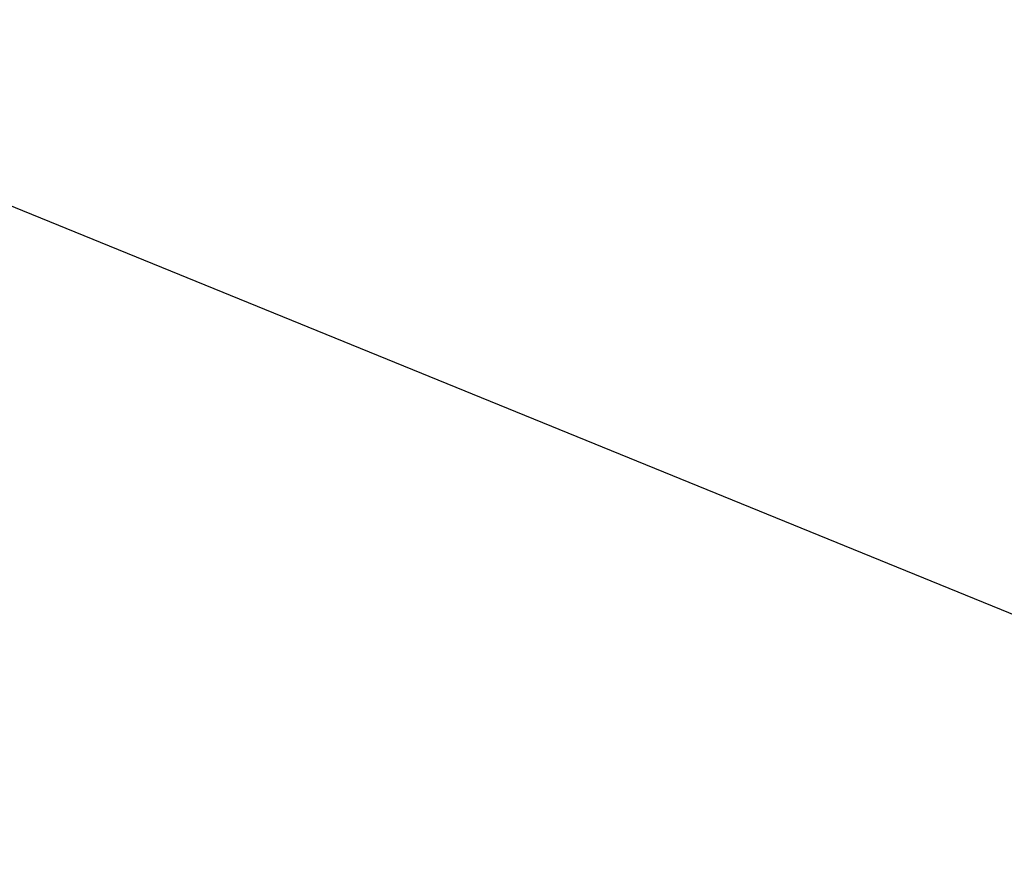
# Model space of a CAD drawing. Units: metres. Extents: x 4298.5 to 4325.2, y 2075 to 2095.8.
# Tile 22 of 35: x 4318.3 to 4320.1, y 2076.7 to 2078.2. Entities that reach past the tile are written whole.
import ezdxf

# ---------------------------------------------------------------- set-up
doc = ezdxf.new("R2010")
doc.units = ezdxf.units.M
doc.layers.add('A-ANNO-DIMS', color=2, linetype='Continuous', lineweight=18)
doc.styles.get("Standard").update_dxf_attribs({"font": 'arial.ttf'})
doc.dimstyles.get("Standard").update_dxf_attribs({"dimtxt": 0.18, "dimasz": 0.18, "dimexe": 0.18, "dimexo": 0.0625, "dimgap": 0.09, "dimtad": 0, "dimtih": 1, "dimtoh": 1, "dimdec": 4, "dimzin": 0, "dimdsep": 46, "dimtxsty": 'Standard', "dimcen": 0.09, "dimadec": 0, "dimazin": 0, "dimtfac": 1, "dimtdec": 4, "dimtofl": 0, "dimtmove": 0, "dimatfit": 3, "dimfxl": 1, "dimtolj": 1, "dimtzin": 0, "dimarcsym": 0})

# ---------------------------------------------------------------- blocks, each defined once
blk = doc.blocks.new('*D47')
at = {"layer": 'A-ANNO-DIMS', "color": 0, "lineweight": -2, "transparency": 16777216}
for p, q in [((4300.4306, 2084.4956), (4300.4306, 2074.9896)), ((4322.8106, 2084.4956), (4322.8106, 2074.9896)), ((4300.6106, 2075.1696), (4311.2252, 2075.1696)), ((4322.6306, 2075.1696), (4312.016, 2075.1696))]:
    blk.add_line(p, q, dxfattribs=at)
at = {"layer": 'A-ANNO-DIMS', "color": 0, "transparency": 16777216}
for points in [[(4300.6106, 2075.1996), (4300.6106, 2075.1396), (4300.4306, 2075.1696)], [(4322.6306, 2075.1996), (4322.6306, 2075.1396), (4322.8106, 2075.1696)]]:
    blk.add_solid(points, dxfattribs=at)
at = {"layer": 'Defpoints', "color": 0, "transparency": 16777216}
for p in [(4300.4306, 2084.5581), (4322.8106, 2084.5581), (4322.8106, 2075.1696)]:
    blk.add_point(p, dxfattribs=at)
at = {"layer": 'A-ANNO-DIMS', "color": 0, "transparency": 16777216, "insert": (4311.6206, 2075.1696), "char_height": 0.18, "attachment_point": 5}
blk.add_mtext('\\A1;22.38', dxfattribs=at)
blk = doc.blocks.new('*D48')
at = {"layer": 'A-ANNO-DIMS', "color": 0, "lineweight": -2, "transparency": 16777216}
for p, q in [((4310.1831, 2094.4781), (4324.7671, 2094.4781)), ((4324.5871, 2094.2981), (4324.5871, 2085.585)), ((4324.5871, 2076.5081), (4324.5871, 2085.2212)), ((4316.8731, 2076.3281), (4324.7671, 2076.3281))]:
    blk.add_line(p, q, dxfattribs=at)
at = {"layer": 'A-ANNO-DIMS', "color": 0, "transparency": 16777216}
for points in [[(4324.5571, 2094.2981), (4324.6171, 2094.2981), (4324.5871, 2094.4781)], [(4324.5571, 2076.5081), (4324.6171, 2076.5081), (4324.5871, 2076.3281)]]:
    blk.add_solid(points, dxfattribs=at)
at = {"layer": 'Defpoints', "color": 0, "transparency": 16777216}
for p in [(4310.1206, 2094.4781), (4316.8106, 2076.3281), (4324.5871, 2076.3281)]:
    blk.add_point(p, dxfattribs=at)
at = {"layer": 'A-ANNO-DIMS', "color": 0, "transparency": 16777216, "insert": (4324.5871, 2085.4031), "char_height": 0.18, "attachment_point": 5}
blk.add_mtext('\\A1;18.15', dxfattribs=at)
blk = doc.blocks.new('*D79')
at = {"layer": 'A-ANNO-DIMS', "color": 0, "lineweight": -2, "transparency": 16777216}
for p, q in [((4313.4743, 2079.7393), (4313.4743, 2079.9193)), ((4313.3843, 2079.8293), (4313.5643, 2079.8293)), ((4320.4622, 2076.981), (4318.0084, 2077.9812)), ((4320.6422, 2076.981), (4320.4622, 2076.981))]:
    blk.add_line(p, q, dxfattribs=at)
at = {"layer": 'A-ANNO-DIMS', "color": 0, "transparency": 16777216}
blk.add_solid([(4318.0197, 2078.009), (4317.9971, 2077.9534), (4317.8417, 2078.0491)], dxfattribs=at)
at = {"layer": 'Defpoints', "color": 0, "transparency": 16777216}
for p in [(4313.4743, 2079.8293), (4317.8417, 2078.0491)]:
    blk.add_point(p, dxfattribs=at)
at = {"layer": 'A-ANNO-DIMS', "color": 0, "transparency": 16777216, "insert": (4321.3169, 2076.981), "char_height": 0.18, "attachment_point": 5}
blk.add_mtext('\\A1;2X R4.716', dxfattribs=at)

msp = doc.modelspace()

# ---------------------------------------------------------------- dimensions: what is measured, and where the dimension line sits
at = {"layer": 'A-ANNO-DIMS'}
dim = msp.add_linear_dim(base=(4324.5871, 2076.3281), p1=(4310.1206, 2094.4781), p2=(4316.8106, 2076.3281), angle=90, dimstyle='Standard', override={"dimdec": 2, "dimlfac": 1, "dimrnd": 0, "dimzin": 0, "dimdsep": 46, "dimlunit": 2}, dxfattribs=at)
dim.commit()
dim.dimension.update_dxf_attribs({"geometry": '*D48', "text_midpoint": (4324.5871, 2085.4031)})
dim = msp.add_linear_dim(base=(4322.8106, 2075.1696), p1=(4300.4306, 2084.5581), p2=(4322.8106, 2084.5581), dimstyle='Standard', override={"dimdec": 2, "dimlfac": 1, "dimrnd": 0, "dimzin": 0, "dimdsep": 46, "dimlunit": 2}, dxfattribs=at)
dim.commit()
dim.dimension.update_dxf_attribs({"geometry": '*D47', "text_midpoint": (4311.6206, 2075.1696)})
dim = msp.add_radius_dim(center=(4313.4743, 2079.8293), mpoint=(4317.8417, 2078.0491), text='2X <>', dimstyle='Standard', override={"dimdec": 3, "dimlfac": 1, "dimrnd": 0, "dimzin": 0, "dimdsep": 46, "dimlunit": 2}, dxfattribs=at)
dim.commit()
dim.dimension.update_dxf_attribs({"geometry": '*D79', "text_midpoint": (4321.3169, 2076.981), "dimtype": 164})

doc.saveas('drawing.dxf')
